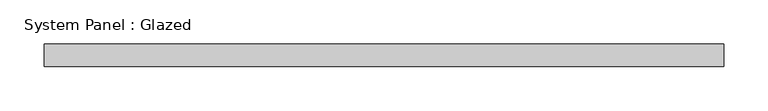
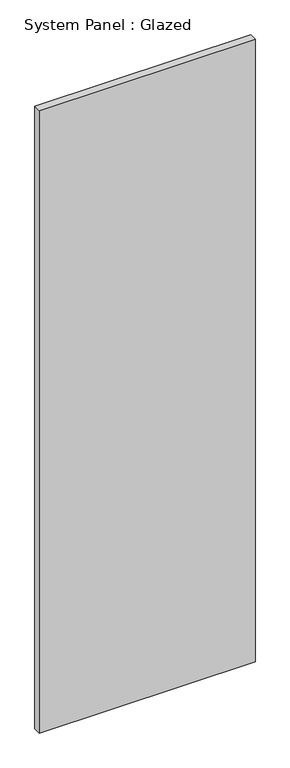
"""IFC4 building model written with IfcOpenShell, lengths in millimetres: plate geometry, System Panel : Glazed."""

from ifc_helpers import new_model, si_unit, origin, origin_with_axes, place, context, project, spatial, polyline, outline, extrude, source, transform, mapped, element, save


def system_panel_glazed_c39fb08b(model_context):
    return source(origin(), model_context, "Body", "SweptSolid", [
        extrude(outline(polyline([(384.175, 19.05), (-384.175, 19.05), (-384.175, 44.45), (384.175, 44.45), (384.175, 19.05)])), origin_with_axes(), (0.0, 0.0, 1.0), 2341.3449309),
    ])


if __name__ == "__main__":
    model = new_model("IFC4")
    model_context = context("Model", 3, world=origin())
    ifc_project = project(units=[si_unit("LENGTHUNIT", "METRE", prefix="MILLI")], contexts=[model_context])
    site = spatial("IfcSite", under=ifc_project)
    building = spatial("IfcBuilding", under=site)
    placement = place(None, origin())
    system_panel_glazed_shape = system_panel_glazed_c39fb08b(model_context)
    element("IfcPlate", 1, ObjectType="System Panel : Glazed", at=placement, inside=building, context=model_context, shape_type="MappedRepresentation", body=[
        mapped(system_panel_glazed_shape, transform((0.0, 0.0, 0.0), x_axis=(1.0, 0.0, 0.0), y_axis=(0.0, 1.0, 0.0), z_axis=(0.0, 0.0, 1.0))),
    ])
    save(model, "model.ifc")

# Revit data of these elements
# Type "System Panel : Glazed"
#   Construction Type Id = "GSP4R"
#   Analytic Construction = "1/8 in Pilkington single glazing"
#   Visual Light Transmittance = 0.9
#   Solar Heat Gain Coefficient = 0.86
#   Heat Transfer Coefficient (U) = 1.18115 BTU/(h·ft²·°F)
#   Define Thermal Properties by = 1
# Element 1 (IfcPlate, "System Panel : Glazed")
#   Materials on its faces: "Glass"
# Materials
#   "Glass": class "Glass", colour RGB 0 128 192, transparency 0.75, Description = "Soda Lime Glass", Cost = 0
